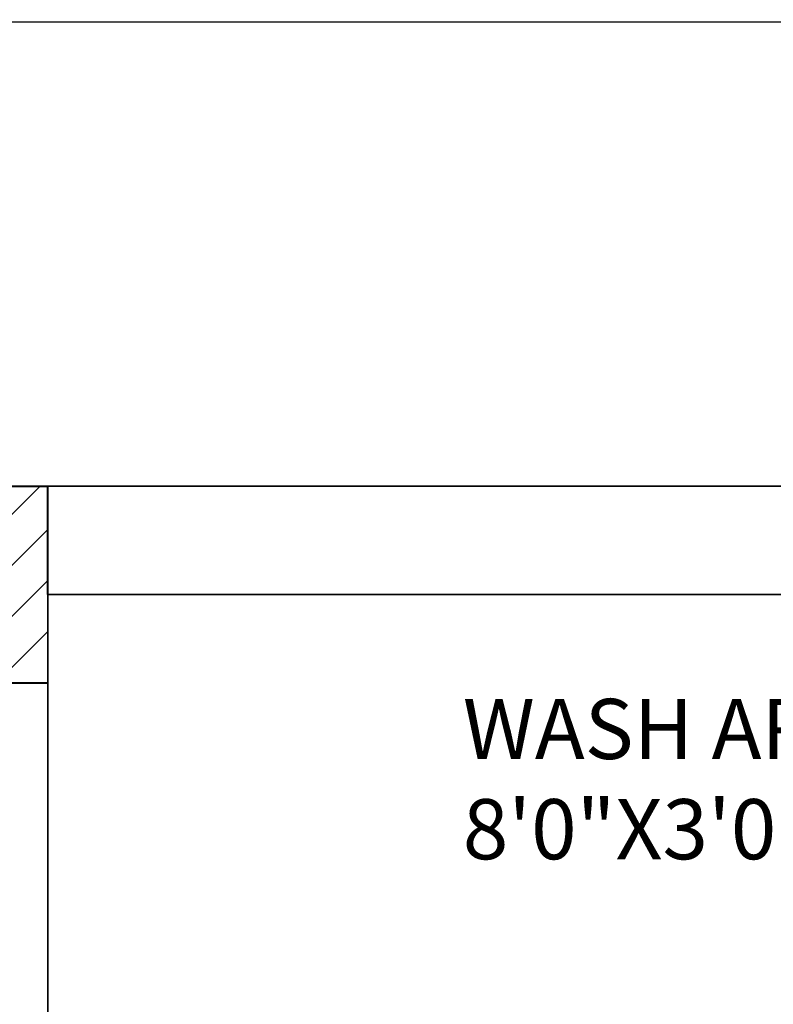
# Model space of a CAD drawing. Units: inches. Extents: x -86 to 2463, y -1058 to 68.
# Tile 15 of 17: x 22 to 85, y -14 to 68. Entities that reach past the tile are written whole.
import ezdxf

# ---------------------------------------------------------------- set-up
doc = ezdxf.new("R2010")
doc.units = ezdxf.units.IN
doc.header["$MEASUREMENT"] = 0
for name, color, linetype, lineweight in [('A-ANNO-DIMS', 2, 'Continuous', 18), ('A-AREA-IDEN', 7, 'Continuous', 18), ('A-COLS', 7, 'Continuous', 40), ('A-COLS-PATT', 252, 'Continuous', 13), ('A-WALL', 7, 'Continuous', 35)]:
    doc.layers.add(name, color=color, linetype=linetype, lineweight=lineweight)
doc.styles.get("Standard").update_dxf_attribs({"font": 'arial.ttf'})
doc.dimstyles.get("Standard").update_dxf_attribs({"dimtxt": 0.18, "dimasz": 0.18, "dimexe": 0.18, "dimexo": 0.0625, "dimgap": 0.09, "dimtad": 0, "dimtih": 1, "dimtoh": 1, "dimdec": 4, "dimzin": 0, "dimdsep": 46, "dimtxsty": 'Standard', "dimcen": 0.09, "dimadec": 0, "dimazin": 0, "dimtfac": 1, "dimtdec": 4, "dimtofl": 0, "dimtmove": 0, "dimatfit": 3, "dimfxl": 1, "dimtolj": 1, "dimtzin": 0, "dimarcsym": 0})

# ---------------------------------------------------------------- blocks, each defined once
blk = doc.blocks.new('*D35')
at = {"layer": 'A-ANNO-DIMS', "color": 0, "lineweight": -2, "transparency": 16777216}
for p, q in [((15.761, 28.958), (15.761, 67.676)), ((15.941, 67.496), (200.989, 67.496)), ((386.581, 67.496), (201.532, 67.496)), ((386.761, 28.958), (386.761, 67.676))]:
    blk.add_line(p, q, dxfattribs=at)
at = {"layer": 'A-ANNO-DIMS', "color": 0, "transparency": 16777216}
for points in [[(15.941, 67.526), (15.941, 67.466), (15.761, 67.496)], [(386.581, 67.526), (386.581, 67.466), (386.761, 67.496)]]:
    blk.add_solid(points, dxfattribs=at)
at = {"layer": 'Defpoints', "color": 0, "transparency": 16777216}
for p in [(386.761, 67.496), (15.761, 28.896), (386.761, 28.896)]:
    blk.add_point(p, dxfattribs=at)
at = {"layer": 'A-ANNO-DIMS', "color": 0, "transparency": 16777216, "insert": (201.261, 67.496), "char_height": 0.18, "attachment_point": 5}
blk.add_mtext('\\A1;371', dxfattribs=at)

msp = doc.modelspace()

# ---------------------------------------------------------------- hatches: boundary and pattern name
at = {"layer": 'A-COLS-PATT'}
h = msp.add_hatch(dxfattribs=at)
h.set_pattern_fill('ANSI31', color=256, scale=24)
h.set_pattern_definition([(45, (-1015.1314, -586.0864), (-2.1213203, 2.1213203), [])])
h.paths.add_polyline_path([(24.761, -294.104), (24.761, -284.978), (15.761, -284.978), (15.761, -303.104), (24.761, -303.104)])
h.paths.add_polyline_path([(199.1, -294.104), (183.761, -294.104), (183.761, -303.104), (199.1, -303.104)])
h.paths.add_polyline_path([(386.761, -294.104), (377.761, -294.104), (369.914, -294.104), (369.914, -303.104), (377.846, -303.104), (386.761, -303.104)])
h.paths.add_polyline_path([(386.761, -145.104), (386.761, -141.104), (377.761, -141.104), (377.761, -145.104), (377.761, -154.61), (386.761, -154.61)])
h.paths.add_polyline_path([(386.761, -154.61), (377.761, -154.61), (377.761, -162.891), (386.761, -162.891)])
h.paths.add_polyline_path([(24.761, -145.104), (24.761, -141.104), (15.761, -141.104), (15.761, -156.678), (24.761, -156.678)])
h.paths.add_polyline_path([(-38.239, 28.896), (-47.239, 28.896), (-47.239, 19.896), (-47.239, 12.652), (-38.239, 12.652), (-38.239, 19.896)])
h.paths.add_polyline_path([(24.761, 28.896), (15.761, 28.896), (15.761, 19.896), (15.761, 12.545), (24.761, 12.545), (24.761, 19.896)])
h.paths.add_polyline_path([(183.507, 19.896), (161.036, 19.896), (161.036, 17.001), (183.507, 17.001)])
h.paths.add_polyline_path([(183.507, 28.896), (161.036, 28.896), (161.036, 19.896), (183.507, 19.896)])
h.paths.add_polyline_path([(386.761, 28.896), (373.166, 28.896), (373.166, 19.896), (377.761, 19.896), (386.761, 19.896)])

# ---------------------------------------------------------------- linework, layer by layer
at = {"layer": 'A-COLS'}
for p, q in [((15.761, 28.896), (24.761, 28.896)), ((24.761, 19.896), (24.761, 28.896)), ((15.761, 12.545), (24.761, 12.545))]:
    msp.add_line(p, q, dxfattribs=at)
at = {"layer": 'A-WALL'}
for p, q in [((24.761, 28.896), (120.761, 28.896)), ((24.761, 19.896), (120.761, 19.896)), ((24.761, -16.104), (24.761, 19.896))]:
    msp.add_line(p, q, dxfattribs=at)

# ---------------------------------------------------------------- texts
at = {"layer": 'A-AREA-IDEN', "insert": (59.281, 11.211), "char_height": 5, "attachment_point": 1}
msp.add_mtext_dynamic_manual_height_columns('WASH AREA\\P8\'0"X3\'0"', width=81.49318, gutter_width=25, heights=[0], dxfattribs=at)

# ---------------------------------------------------------------- dimensions: what is measured, and where the dimension line sits
at = {"layer": 'A-ANNO-DIMS'}
dim = msp.add_linear_dim(base=(386.761, 67.496), p1=(15.761, 28.896), p2=(386.761, 28.896), dimstyle='Standard', override={"dimdec": 0, "dimlfac": 1, "dimrnd": 0, "dimzin": 0, "dimdsep": 46, "dimlunit": 2}, dxfattribs=at)
dim.commit()
dim.dimension.update_dxf_attribs({"geometry": '*D35', "text_midpoint": (201.261, 67.496)})

doc.saveas('drawing.dxf')
